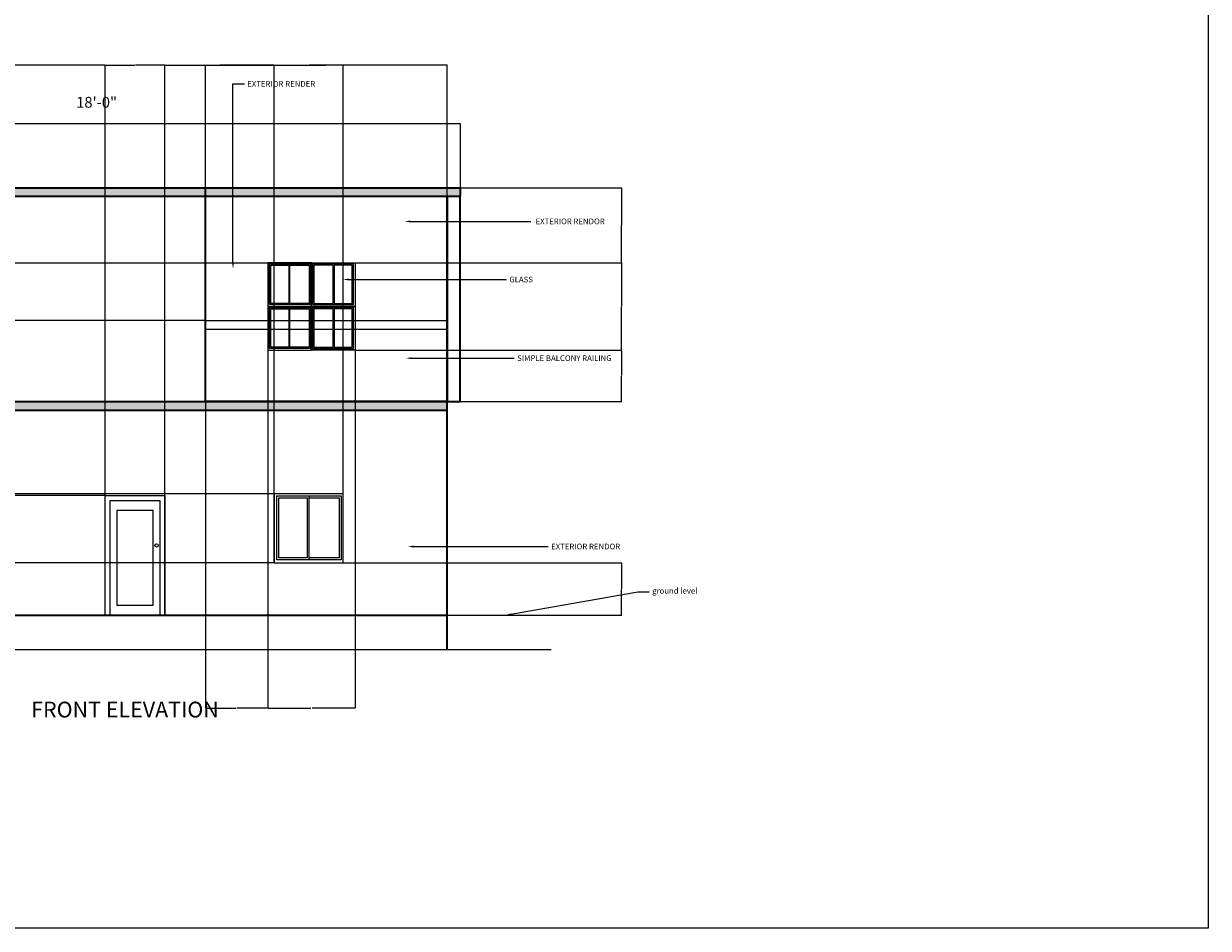
# Model space of a CAD drawing. Units: feet. Extents: x 2813 to 4435, y 1041 to 2557.
# Tile 4 of 6: x 3605 to 4435, y 1041 to 1676. Entities that reach past the tile are written whole.
import ezdxf
from ezdxf import colors
from ezdxf.entities.mleader import LeaderData, LeaderLine
from ezdxf.math import Vec2, Vec3

# ---------------------------------------------------------------- set-up
doc = ezdxf.new("R2010")
doc.units = ezdxf.units.FT
for name, color, linetype, lineweight in [('A-ANNO-DIMS', 2, 'Continuous', 18), ('A-ANNO-SYMB', 7, 'Continuous', 18), ('A-ANNO-TEXT', 7, 'Continuous', 18), ('A-ANNO-TTLB', 7, 'Continuous', 25), ('A-DOOR', 3, 'Continuous', 25), ('A-ELEV', 7, 'Continuous', 35), ('A-ELEV-GRND', 7, 'Continuous', 25), ('A-ELEV-PATT', 252, 'Continuous', 13), ('A-FLOR-HRAL', 4, 'Continuous', 18), ('A-GLAZ', 4, 'Continuous', 18)]:
    doc.layers.add(name, color=color, linetype=linetype, lineweight=lineweight)
doc.styles.get("Standard").update_dxf_attribs({"font": 'arial.ttf'})
doc.dimstyles.get("Standard").update_dxf_attribs({"dimtxt": 0.18, "dimasz": 0.18, "dimexe": 0.18, "dimexo": 0.0625, "dimgap": 0.09, "dimtad": 0, "dimtih": 1, "dimtoh": 1, "dimdec": 4, "dimzin": 0, "dimdsep": 46, "dimtxsty": 'Standard', "dimcen": 0.09, "dimadec": 0, "dimazin": 0, "dimtfac": 1, "dimtdec": 4, "dimtofl": 0, "dimtmove": 0, "dimatfit": 3, "dimfxl": 1, "dimtolj": 1, "dimtzin": 0, "dimarcsym": 0})

# ---------------------------------------------------------------- blocks, each defined once
blk = doc.blocks.new('*U12')
blk.add_lwpolyline([(3.12, 0.01), (0.12, 0.01), (0.12, 72.01), (36.12, 72.01), (36.12, 0.01), (33.12, 0.01)])
for points in [[(33.12, 68.99), (33.12, 0.01), (3.12, 0.01), (3.12, 68.99)], [(29.12, 6.01), (29.12, 62.99), (7.12, 62.99), (7.12, 6.01)]]:
    blk.add_lwpolyline(points, close=True)
blk.add_circle((31.12, 42.01), 1)
blk = doc.blocks.new('*U14')
for p, q in [((38.1, 38.1), (38.1, 876.3)), ((38.1, 876.3), (457.2, 876.3)), ((457.2, 38.1), (457.2, 876.3)), ((457.2, 876.3), (876.3, 876.3)), ((876.3, 876.3), (876.3, 38.1)), ((457.2, 38.1), (38.1, 38.1)), ((876.3, 38.1), (457.2, 38.1))]:
    blk.add_line(p, q)
blk.add_lwpolyline([(0, 0), (900, 0), (900, 900), (0, 900)], close=True)
for points in [[(431.8, 850.9), (431.8, 63.5), (63.5, 63.5), (63.5, 850.9), (431.8, 850.9)], [(457.2, 850.9), (850.9, 850.9), (850.9, 63.5), (457.2, 63.5)]]:
    blk.add_lwpolyline(points)
blk = doc.blocks.new('*D35')
at = {"layer": 'A-ANNO-DIMS', "color": 0, "lineweight": -2, "transparency": 16777216}
for p, q in [((3421.71, 1261.18), (3421.71, 1647.39)), ((3421.89, 1647.21), (3541.42, 1647.21)), ((3661.53, 1647.21), (3542, 1647.21)), ((3661.71, 1261.18), (3661.71, 1647.39))]:
    blk.add_line(p, q, dxfattribs=at)
at = {"layer": 'A-ANNO-DIMS', "color": 0, "transparency": 16777216}
for points in [[(3421.89, 1647.24), (3421.89, 1647.18), (3421.71, 1647.21)], [(3661.53, 1647.24), (3661.53, 1647.18), (3661.71, 1647.21)]]:
    blk.add_solid(points, dxfattribs=at)
at = {"layer": 'DEFPOINTS', "color": 0, "transparency": 16777216}
for p in [(3661.71, 1647.21), (3421.71, 1261.11), (3661.71, 1261.11)]:
    blk.add_point(p, dxfattribs=at)
at = {"layer": 'A-ANNO-DIMS', "color": 0, "transparency": 16777216, "insert": (3541.71, 1647.21), "char_height": 0.18, "attachment_point": 5}
blk.add_mtext('\\A1;240', dxfattribs=at)
blk = doc.blocks.new('*D36')
at = {"layer": 'A-ANNO-DIMS', "color": 0, "lineweight": -2, "transparency": 16777216}
for p, q in [((3661.71, 1345.18), (3661.71, 1647.39)), ((3661.89, 1647.21), (3682.48, 1647.21)), ((3703.53, 1647.21), (3682.93, 1647.21)), ((3703.71, 1345.18), (3703.71, 1647.39))]:
    blk.add_line(p, q, dxfattribs=at)
at = {"layer": 'A-ANNO-DIMS', "color": 0, "transparency": 16777216}
for points in [[(3661.89, 1647.24), (3661.89, 1647.18), (3661.71, 1647.21)], [(3703.53, 1647.24), (3703.53, 1647.18), (3703.71, 1647.21)]]:
    blk.add_solid(points, dxfattribs=at)
at = {"layer": 'DEFPOINTS', "color": 0, "transparency": 16777216}
for p in [(3703.71, 1647.21), (3661.71, 1345.11), (3703.71, 1345.11)]:
    blk.add_point(p, dxfattribs=at)
at = {"layer": 'A-ANNO-DIMS', "color": 0, "transparency": 16777216, "insert": (3682.71, 1647.21), "char_height": 0.18, "attachment_point": 5}
blk.add_mtext('\\A1;42', dxfattribs=at)
blk = doc.blocks.new('*D37')
at = {"layer": 'A-ANNO-DIMS', "color": 0, "lineweight": -2, "transparency": 16777216}
for p, q in [((3703.71, 1261.18), (3703.71, 1647.39)), ((3703.89, 1647.21), (3741.63, 1647.21)), ((3780.03, 1647.21), (3742.28, 1647.21)), ((3780.21, 1297.98), (3780.21, 1647.39))]:
    blk.add_line(p, q, dxfattribs=at)
at = {"layer": 'A-ANNO-DIMS', "color": 0, "transparency": 16777216}
for points in [[(3703.89, 1647.24), (3703.89, 1647.18), (3703.71, 1647.21)], [(3780.03, 1647.24), (3780.03, 1647.18), (3780.21, 1647.21)]]:
    blk.add_solid(points, dxfattribs=at)
at = {"layer": 'DEFPOINTS', "color": 0, "transparency": 16777216}
for p in [(3780.21, 1647.21), (3780.21, 1297.91), (3703.71, 1261.11)]:
    blk.add_point(p, dxfattribs=at)
at = {"layer": 'A-ANNO-DIMS', "color": 0, "transparency": 16777216, "insert": (3741.96, 1647.21), "char_height": 0.18, "attachment_point": 5}
blk.add_mtext('\\A1;76.5', dxfattribs=at)
blk = doc.blocks.new('*D38')
at = {"layer": 'A-ANNO-DIMS', "color": 0, "lineweight": -2, "transparency": 16777216}
for p, q in [((3780.21, 1346.36), (3780.21, 1647.39)), ((3780.39, 1647.21), (3804, 1647.21)), ((3828.4, 1647.21), (3804.79, 1647.21)), ((3828.58, 1346.36), (3828.58, 1647.39))]:
    blk.add_line(p, q, dxfattribs=at)
at = {"layer": 'A-ANNO-DIMS', "color": 0, "transparency": 16777216}
for points in [[(3780.39, 1647.24), (3780.39, 1647.18), (3780.21, 1647.21)], [(3828.4, 1647.24), (3828.4, 1647.18), (3828.58, 1647.21)]]:
    blk.add_solid(points, dxfattribs=at)
at = {"layer": 'DEFPOINTS', "color": 0, "transparency": 16777216}
for p in [(3828.58, 1647.21), (3780.21, 1346.29), (3828.58, 1346.29)]:
    blk.add_point(p, dxfattribs=at)
at = {"layer": 'A-ANNO-DIMS', "color": 0, "transparency": 16777216, "insert": (3804.39, 1647.21), "char_height": 0.18, "attachment_point": 5}
blk.add_mtext('\\A1;48.38', dxfattribs=at)
blk = doc.blocks.new('*D41')
at = {"layer": 'A-ANNO-DIMS', "color": 0, "lineweight": -2, "transparency": 16777216}
for p, q in [((3775.79, 1447.05), (3775.79, 1195.88)), ((3732.18, 1411.05), (3732.18, 1195.88)), ((3732.36, 1196.06), (3753.61, 1196.06)), ((3775.61, 1196.06), (3754.37, 1196.06))]:
    blk.add_line(p, q, dxfattribs=at)
at = {"layer": 'A-ANNO-DIMS', "color": 0, "transparency": 16777216}
for points in [[(3732.36, 1196.09), (3732.36, 1196.03), (3732.18, 1196.06)], [(3775.61, 1196.09), (3775.61, 1196.03), (3775.79, 1196.06)]]:
    blk.add_solid(points, dxfattribs=at)
at = {"layer": 'DEFPOINTS', "color": 0, "transparency": 16777216}
for p in [(3775.79, 1447.11), (3732.18, 1411.11), (3775.79, 1196.06)]:
    blk.add_point(p, dxfattribs=at)
at = {"layer": 'A-ANNO-DIMS', "color": 0, "transparency": 16777216, "insert": (3753.99, 1196.06), "char_height": 0.18, "attachment_point": 5}
blk.add_mtext('\\A1;43.61', dxfattribs=at)
blk = doc.blocks.new('*D42')
at = {"layer": 'A-ANNO-DIMS', "color": 0, "lineweight": -2, "transparency": 16777216}
for p, q in [((3775.79, 1447.05), (3775.79, 1195.88)), ((3837.14, 1447.05), (3837.14, 1195.88)), ((3775.97, 1196.06), (3806.07, 1196.06)), ((3836.96, 1196.06), (3806.86, 1196.06))]:
    blk.add_line(p, q, dxfattribs=at)
at = {"layer": 'A-ANNO-DIMS', "color": 0, "transparency": 16777216}
for points in [[(3775.97, 1196.09), (3775.97, 1196.03), (3775.79, 1196.06)], [(3836.96, 1196.09), (3836.96, 1196.03), (3837.14, 1196.06)]]:
    blk.add_solid(points, dxfattribs=at)
at = {"layer": 'DEFPOINTS', "color": 0, "transparency": 16777216}
for p in [(3775.79, 1447.11), (3837.14, 1447.11), (3837.14, 1196.06)]:
    blk.add_point(p, dxfattribs=at)
at = {"layer": 'A-ANNO-DIMS', "color": 0, "transparency": 16777216, "insert": (3806.46, 1196.06), "char_height": 0.18, "attachment_point": 5}
blk.add_mtext('\\A1;61.35', dxfattribs=at)
blk = doc.blocks.new('*D43')
at = {"layer": 'A-ANNO-DIMS', "color": 0, "lineweight": -2, "transparency": 16777216}
for p, q in [((3661.64, 1345.11), (3260.3, 1345.11)), ((3260.48, 1344.93), (3260.48, 1303.3)), ((3260.48, 1261.29), (3260.48, 1302.93)), ((3661.64, 1261.11), (3260.3, 1261.11))]:
    blk.add_line(p, q, dxfattribs=at)
at = {"layer": 'A-ANNO-DIMS', "color": 0, "transparency": 16777216}
for points in [[(3260.45, 1344.93), (3260.51, 1344.93), (3260.48, 1345.11)], [(3260.45, 1261.29), (3260.51, 1261.29), (3260.48, 1261.11)]]:
    blk.add_solid(points, dxfattribs=at)
at = {"layer": 'DEFPOINTS', "color": 0, "transparency": 16777216}
for p in [(3260.48, 1345.11), (3661.71, 1345.11), (3661.71, 1261.11)]:
    blk.add_point(p, dxfattribs=at)
at = {"layer": 'A-ANNO-DIMS', "color": 0, "transparency": 16777216, "insert": (3260.48, 1303.11), "char_height": 0.18, "attachment_point": 5}
blk.add_mtext('\\A1;84', dxfattribs=at)
blk = doc.blocks.new('*D44')
at = {"layer": 'A-ANNO-DIMS', "color": 0, "lineweight": -2, "transparency": 16777216}
for p, q in [((3780.27, 1297.91), (4024.11, 1297.91)), ((4023.93, 1297.73), (4023.93, 1279.7)), ((4023.93, 1261.29), (4023.93, 1279.33)), ((3703.77, 1261.11), (4024.11, 1261.11))]:
    blk.add_line(p, q, dxfattribs=at)
at = {"layer": 'A-ANNO-DIMS', "color": 0, "transparency": 16777216}
for points in [[(4023.9, 1297.73), (4023.96, 1297.73), (4023.93, 1297.91)], [(4023.9, 1261.29), (4023.96, 1261.29), (4023.93, 1261.11)]]:
    blk.add_solid(points, dxfattribs=at)
at = {"layer": 'DEFPOINTS', "color": 0, "transparency": 16777216}
for p in [(3780.21, 1297.91), (4023.93, 1297.91), (3703.71, 1261.11)]:
    blk.add_point(p, dxfattribs=at)
at = {"layer": 'A-ANNO-DIMS', "color": 0, "transparency": 16777216, "insert": (4023.93, 1279.51), "char_height": 0.18, "attachment_point": 5}
blk.add_mtext('\\A1;36.8', dxfattribs=at)
blk = doc.blocks.new('*D45')
at = {"layer": 'A-ANNO-DIMS', "color": 0, "lineweight": -2, "transparency": 16777216}
for p, q in [((3780.14, 1346.29), (3260.3, 1346.29)), ((3260.48, 1346.11), (3260.48, 1322.29)), ((3260.48, 1298.09), (3260.48, 1321.92)), ((3780.14, 1297.91), (3260.3, 1297.91))]:
    blk.add_line(p, q, dxfattribs=at)
at = {"layer": 'A-ANNO-DIMS', "color": 0, "transparency": 16777216}
for points in [[(3260.45, 1346.11), (3260.51, 1346.11), (3260.48, 1346.29)], [(3260.45, 1298.09), (3260.51, 1298.09), (3260.48, 1297.91)]]:
    blk.add_solid(points, dxfattribs=at)
at = {"layer": 'DEFPOINTS', "color": 0, "transparency": 16777216}
for p in [(3260.48, 1346.29), (3780.21, 1346.29), (3780.21, 1297.91)]:
    blk.add_point(p, dxfattribs=at)
at = {"layer": 'A-ANNO-DIMS', "color": 0, "transparency": 16777216, "insert": (3260.48, 1322.1), "char_height": 0.18, "attachment_point": 5}
blk.add_mtext('\\A1;48.38', dxfattribs=at)
blk = doc.blocks.new('*D47')
at = {"layer": 'A-ANNO-DIMS', "color": 0, "lineweight": -2, "transparency": 16777216}
for p, q in [((3421.77, 1561.11), (4024.11, 1561.11)), ((4023.93, 1560.93), (4023.93, 1534.97)), ((4023.93, 1508.64), (4023.93, 1534.61)), ((3480.84, 1508.46), (4024.11, 1508.46))]:
    blk.add_line(p, q, dxfattribs=at)
at = {"layer": 'A-ANNO-DIMS', "color": 0, "transparency": 16777216}
for points in [[(4023.9, 1560.93), (4023.96, 1560.93), (4023.93, 1561.11)], [(4023.9, 1508.64), (4023.96, 1508.64), (4023.93, 1508.46)]]:
    blk.add_solid(points, dxfattribs=at)
at = {"layer": 'DEFPOINTS', "color": 0, "transparency": 16777216}
for p in [(3421.71, 1561.11), (3480.78, 1508.46), (4023.93, 1508.46)]:
    blk.add_point(p, dxfattribs=at)
at = {"layer": 'A-ANNO-DIMS', "color": 0, "transparency": 16777216, "insert": (4023.93, 1534.79), "char_height": 0.18, "attachment_point": 5}
blk.add_mtext('\\A1;52.65', dxfattribs=at)
blk = doc.blocks.new('*D48')
at = {"layer": 'A-ANNO-DIMS', "color": 0, "lineweight": -2, "transparency": 16777216}
for p, q in [((3837.2, 1508.46), (4024.11, 1508.46)), ((4023.93, 1508.28), (4023.93, 1477.97)), ((4023.93, 1447.29), (4023.93, 1477.61)), ((3837.2, 1447.11), (4024.11, 1447.11))]:
    blk.add_line(p, q, dxfattribs=at)
at = {"layer": 'A-ANNO-DIMS', "color": 0, "transparency": 16777216}
for points in [[(4023.9, 1508.28), (4023.96, 1508.28), (4023.93, 1508.46)], [(4023.9, 1447.29), (4023.96, 1447.29), (4023.93, 1447.11)]]:
    blk.add_solid(points, dxfattribs=at)
at = {"layer": 'DEFPOINTS', "color": 0, "transparency": 16777216}
for p in [(3837.14, 1508.46), (4023.93, 1508.46), (3837.14, 1447.11)]:
    blk.add_point(p, dxfattribs=at)
at = {"layer": 'A-ANNO-DIMS', "color": 0, "transparency": 16777216, "insert": (4023.93, 1477.79), "char_height": 0.18, "attachment_point": 5}
blk.add_mtext('\\A1;61.35', dxfattribs=at)
blk = doc.blocks.new('*D49')
at = {"layer": 'A-ANNO-DIMS', "color": 0, "lineweight": -2, "transparency": 16777216}
for p, q in [((3732.12, 1467.89), (3260.3, 1467.89)), ((3260.48, 1467.71), (3260.48, 1439.68)), ((3260.48, 1411.29), (3260.48, 1439.32)), ((3732.12, 1411.11), (3260.3, 1411.11))]:
    blk.add_line(p, q, dxfattribs=at)
at = {"layer": 'A-ANNO-DIMS', "color": 0, "transparency": 16777216}
for points in [[(3260.45, 1467.71), (3260.51, 1467.71), (3260.48, 1467.89)], [(3260.45, 1411.29), (3260.51, 1411.29), (3260.48, 1411.11)]]:
    blk.add_solid(points, dxfattribs=at)
at = {"layer": 'DEFPOINTS', "color": 0, "transparency": 16777216}
for p in [(3260.48, 1467.89), (3732.18, 1467.89), (3732.18, 1411.11)]:
    blk.add_point(p, dxfattribs=at)
at = {"layer": 'A-ANNO-DIMS', "color": 0, "transparency": 16777216, "insert": (3260.48, 1439.5), "char_height": 0.18, "attachment_point": 5}
blk.add_mtext('\\A1;56.77', dxfattribs=at)
blk = doc.blocks.new('*D50')
at = {"layer": 'A-ANNO-DIMS', "color": 0, "lineweight": -2, "transparency": 16777216}
for p, q in [((3837.2, 1447.11), (4024.11, 1447.11)), ((4023.93, 1446.93), (4023.93, 1429.3)), ((4023.93, 1411.29), (4023.93, 1428.93)), ((3901.77, 1411.11), (4024.11, 1411.11))]:
    blk.add_line(p, q, dxfattribs=at)
at = {"layer": 'A-ANNO-DIMS', "color": 0, "transparency": 16777216}
for points in [[(4023.9, 1446.93), (4023.96, 1446.93), (4023.93, 1447.11)], [(4023.9, 1411.29), (4023.96, 1411.29), (4023.93, 1411.11)]]:
    blk.add_solid(points, dxfattribs=at)
at = {"layer": 'DEFPOINTS', "color": 0, "transparency": 16777216}
for p in [(3837.14, 1447.11), (4023.93, 1447.11), (3901.71, 1411.11)]:
    blk.add_point(p, dxfattribs=at)
at = {"layer": 'A-ANNO-DIMS', "color": 0, "transparency": 16777216, "insert": (4023.93, 1429.11), "char_height": 0.18, "attachment_point": 5}
blk.add_mtext('\\A1;36', dxfattribs=at)
blk = doc.blocks.new('*D51')
at = {"layer": 'A-ANNO-DIMS', "color": 0, "lineweight": -2, "transparency": 16777216}
for p, q in [((3732.18, 1411.18), (3732.18, 1647.39)), ((3732.36, 1647.21), (3816.49, 1647.21)), ((3901.53, 1647.21), (3817.4, 1647.21)), ((3901.71, 1411.18), (3901.71, 1647.39))]:
    blk.add_line(p, q, dxfattribs=at)
at = {"layer": 'A-ANNO-DIMS', "color": 0, "transparency": 16777216}
for points in [[(3732.36, 1647.24), (3732.36, 1647.18), (3732.18, 1647.21)], [(3901.53, 1647.24), (3901.53, 1647.18), (3901.71, 1647.21)]]:
    blk.add_solid(points, dxfattribs=at)
at = {"layer": 'DEFPOINTS', "color": 0, "transparency": 16777216}
for p in [(3901.71, 1647.21), (3732.18, 1411.11), (3901.71, 1411.11)]:
    blk.add_point(p, dxfattribs=at)
at = {"layer": 'A-ANNO-DIMS', "color": 0, "transparency": 16777216, "insert": (3816.94, 1647.21), "char_height": 0.18, "attachment_point": 5}
blk.add_mtext('\\A1;169.52', dxfattribs=at)

msp = doc.modelspace()

# ---------------------------------------------------------------- hatches: boundary and pattern name
at = {"layer": 'A-ELEV-PATT'}
h = msp.add_hatch(color=256, dxfattribs=at)
h.dxf.hatch_style = 1
h.paths.add_polyline_path([(3732.181, 1561.114), (3421.706, 1561.114), (3421.706, 1555.114), (3732.181, 1555.114)])
h.paths.add_polyline_path([(3910.706, 1561.114), (3901.706, 1561.114), (3751.395, 1561.114), (3751.395, 1555.114), (3901.706, 1555.114), (3910.706, 1555.114)])
h.paths.add_polyline_path([(3751.395, 1561.114), (3732.181, 1561.114), (3732.181, 1555.114), (3751.395, 1555.114)])
h.paths.add_polyline_path([(3421.706, 1561.114), (3374.104, 1561.114), (3374.104, 1555.114), (3421.706, 1555.114)])
h.paths.add_polyline_path([(3901.706, 1411.114), (3732.181, 1411.114), (3421.706, 1411.114), (3421.706, 1405.114), (3901.706, 1405.114)])
h.paths.add_polyline_path([(3421.706, 1411.114), (3374.104, 1411.114), (3374.104, 1405.114), (3421.706, 1405.114)])

# ---------------------------------------------------------------- linework, layer by layer
at = {"layer": 'A-ANNO-DIMS'}
for p, q in [((3374.104, 1606.165), (3910.706, 1606.165)), ((3910.706, 1606.165), (3910.706, 1561.114))]:
    msp.add_line(p, q, dxfattribs=at)
at = {"layer": 'A-ANNO-TTLB'}
for p, q in [((4435.474, 2556.562), (4435.474, 1041.465)), ((4435.474, 1041.465), (2933.466, 1041.465))]:
    msp.add_line(p, q, dxfattribs=at)
at = {"layer": 'A-ELEV'}
for p, q in [((3350.104, 1561.114), (3901.706, 1561.114)), ((3374.104, 1555.114), (3901.706, 1555.114)), ((3732.181, 1555.114), (3732.181, 1561.114)), ((3901.706, 1561.114), (3910.706, 1561.114)), ((3901.706, 1237.114), (3901.706, 1555.114)), ((3901.706, 1411.114), (3901.706, 1555.114)), ((3901.706, 1555.114), (3910.706, 1555.114)), ((3910.706, 1561.114), (3910.706, 1555.114)), ((3910.706, 1411.114), (3910.706, 1555.114)), ((3374.104, 1411.114), (3910.706, 1411.114)), ((3374.104, 1405.114), (3901.706, 1405.114)), ((3421.706, 1261.114), (3901.706, 1261.114))]:
    msp.add_line(p, q, dxfattribs=at)
msp.add_lwpolyline([(3732.181, 1555.114), (3901.706, 1555.114), (3901.706, 1411.114), (3732.181, 1411.114)], close=True, dxfattribs=at)
at = {"layer": 'A-ELEV-GRND'}
for p, q in [((3901.706, 1261.114), (3982.882, 1261.114)), ((3421.706, 1237.114), (3901.706, 1237.114)), ((3901.706, 1237.114), (3974.556, 1237.114))]:
    msp.add_line(p, q, dxfattribs=at)
at = {"layer": 'A-FLOR-HRAL'}
for p, q in [((3732.181, 1467.886), (3901.706, 1467.886)), ((3732.181, 1461.886), (3901.706, 1461.886))]:
    msp.add_line(p, q, dxfattribs=at)

# ---------------------------------------------------------------- block references
at = {"layer": 'A-DOOR', "xscale": 1.166666666666666, "yscale": 1.166666666666666, "zscale": 1.166666666666666}
msp.add_blockref('*U12', (3661.562, 1261.099), dxfattribs=at)
at = {"layer": 'A-GLAZ'}
for p, xscale, yscale, zscale in [((3775.791, 1477.788), 0.0340819276308726, 0.0340819276308726, 0.0340819276308726), ((3837.138, 1477.788), -0.0340819276308726, 0.0340819276308726, 0.0340819276308726), ((3775.791, 1447.114), 0.0340819276308726, 0.0340819276308726, 0.0340819276308726), ((3837.138, 1447.114), -0.0340819276308726, 0.0340819276308726, 0.0340819276308726), ((3780.205, 1297.915), 0.0537544395331253, 0.0537544395331253, 0.0537544395331253)]:
    msp.add_blockref('*U14', p, dxfattribs=dict(at, xscale=xscale, yscale=yscale, zscale=zscale))

# ---------------------------------------------------------------- texts
at = {"layer": 'A-ANNO-DIMS', "insert": (3641.405, 1624.886), "char_height": 7.6018, "attachment_point": 1}
msp.add_mtext_dynamic_manual_height_columns('18\'-0"', width=61.91074, gutter_width=38.009, heights=[0], dxfattribs=at)
at = {"layer": 'A-ANNO-TEXT', "insert": (3609.833, 1200.48), "char_height": 11.04352, "attachment_point": 1}
msp.add_mtext_dynamic_manual_height_columns('FRONT ELEVATION', width=1286.33739, gutter_width=55.218, heights=[0], dxfattribs=at)

# ---------------------------------------------------------------- dimensions: what is measured, and where the dimension line sits
at = {"layer": 'A-ANNO-DIMS'}
for base, p1, p2, override, picture, middle in [((3661.706, 1647.215), (3421.706, 1261.114), (3661.706, 1261.114), {"dimdec": 0, "dimlfac": 1, "dimrnd": 0, "dimzin": 0, "dimdsep": 46, "dimlunit": 2}, '*D35', (3541.706, 1647.215)), ((3703.706, 1647.215), (3661.706, 1345.114), (3703.706, 1345.114), {"dimdec": 0, "dimlfac": 1, "dimrnd": 0, "dimzin": 0, "dimdsep": 46, "dimlunit": 2}, '*D36', (3682.706, 1647.215)), ((3780.205, 1647.215), (3703.706, 1261.114), (3780.205, 1297.915), {"dimdec": 1, "dimlfac": 1, "dimrnd": 0, "dimzin": 0, "dimdsep": 46, "dimlunit": 2}, '*D37', (3741.956, 1647.215)), ((3901.70615, 1647.21469), (3732.18117, 1411.1143), (3901.70615, 1411.1143), {"dimdec": 2, "dimlfac": 1, "dimrnd": 0, "dimzin": 0, "dimdsep": 46, "dimlunit": 2}, '*D51', (3816.94366, 1647.21469)), ((3828.584, 1647.215), (3780.205, 1346.294), (3828.584, 1346.294), {"dimdec": 2, "dimlfac": 1, "dimrnd": 0, "dimzin": 0, "dimdsep": 46, "dimlunit": 2}, '*D38', (3804.395, 1647.215)), ((3775.791, 1196.064), (3732.181, 1411.114), (3775.791, 1447.114), {"dimdec": 2, "dimlfac": 1, "dimrnd": 0, "dimzin": 0, "dimdsep": 46, "dimlunit": 2}, '*D41', (3753.986, 1196.064)), ((3837.138, 1196.064), (3775.791, 1447.114), (3837.138, 1447.114), {"dimdec": 2, "dimlfac": 1, "dimrnd": 0, "dimzin": 0, "dimdsep": 46, "dimlunit": 2}, '*D42', (3806.464, 1196.064))]:
    dim = msp.add_linear_dim(base=base, p1=p1, p2=p2, dimstyle='Standard', override=override, dxfattribs=at)
    dim.commit()
    dim.dimension.update_dxf_attribs({"geometry": picture, "text_midpoint": middle})
for base, p1, p2, override, picture, middle in [((4023.932, 1508.462), (3421.706, 1561.114), (3480.779, 1508.462), {"dimdec": 2, "dimlfac": 1, "dimrnd": 0, "dimzin": 0, "dimdsep": 46, "dimlunit": 2}, '*D47', (4023.932, 1534.788)), ((4023.932, 1508.462), (3837.138, 1447.114), (3837.138, 1508.462), {"dimdec": 2, "dimlfac": 1, "dimrnd": 0, "dimzin": 0, "dimdsep": 46, "dimlunit": 2}, '*D48', (4023.932, 1477.788)), ((3260.476, 1467.886), (3732.181, 1411.114), (3732.181, 1467.886), {"dimdec": 2, "dimlfac": 1, "dimrnd": 0, "dimzin": 0, "dimdsep": 46, "dimlunit": 2}, '*D49', (3260.476, 1439.5)), ((4023.932, 1447.114), (3901.706, 1411.114), (3837.138, 1447.114), {"dimdec": 0, "dimlfac": 1, "dimrnd": 0, "dimzin": 0, "dimdsep": 46, "dimlunit": 2}, '*D50', (4023.932, 1429.114)), ((3260.476, 1346.294), (3780.205, 1297.915), (3780.205, 1346.294), {"dimdec": 2, "dimlfac": 1, "dimrnd": 0, "dimzin": 0, "dimdsep": 46, "dimlunit": 2}, '*D45', (3260.476, 1322.104)), ((3260.476, 1345.114), (3661.706, 1261.114), (3661.706, 1345.114), {"dimdec": 0, "dimlfac": 1, "dimrnd": 0, "dimzin": 0, "dimdsep": 46, "dimlunit": 2}, '*D43', (3260.476, 1303.114)), ((4023.932, 1297.915), (3703.706, 1261.114), (3780.205, 1297.915), {"dimdec": 1, "dimlfac": 1, "dimrnd": 0, "dimzin": 0, "dimdsep": 46, "dimlunit": 2}, '*D44', (4023.932, 1279.514))]:
    dim = msp.add_linear_dim(base=base, p1=p1, p2=p2, angle=90, dimstyle='Standard', override=override, dxfattribs=at)
    dim.commit()
    dim.dimension.update_dxf_attribs({"geometry": picture, "text_midpoint": middle})

# ---------------------------------------------------------------- leaders
at = {"layer": 'A-ANNO-SYMB'}
ml = msp.add_multileader_mtext('Standard', dxfattribs=at)
ml.set_content('ground level', color=256)
ml.set_leader_properties()
ml.build(insert=Vec2(0, 0))
ctx = ml.context
ctx.base_point, ctx.plane_origin = Vec3(4043.415, 1277.694), Vec3(3942.294, 1261.114)
notes = []
notes.append((ctx, [(0, (1, 1, 0), (4035.415, 1277.694), (1, 0), 8, [(0, [(3942.294, 1261.114)], 0, [])])]))
ctx.mtext.insert, ctx.mtext.flow_direction = Vec3(4045.415, 1280.282), 5
at = {"layer": 'A-ANNO-TEXT'}
ml = msp.add_multileader_mtext('Standard', dxfattribs=at)
ml.set_content('EXTERIOR RENDER', color=256)
ml.set_leader_properties()
ml.build(insert=Vec2(0, 0))
ctx = ml.context
ctx.base_point, ctx.plane_origin = Vec3(3759.395, 1633.985), Vec3(3751.395, 1504.33)
notes.append((ctx, [(0, (1, 1, 0), (3751.395, 1633.985), (1, 0), 8, [(0, [(3751.395, 1504.33)], 0, [])])]))
ctx.mtext.insert, ctx.mtext.flow_direction = Vec3(3761.395, 1636.019), 5
ml = msp.add_multileader_mtext('Standard', dxfattribs=at)
ml.set_content(' EXTERIOR RENDOR', color=256)
ml.set_leader_properties()
ml.build(insert=Vec2(0, 0))
ctx = ml.context
ctx.base_point, ctx.plane_origin = Vec3(3960.376, 1537.496), Vec3(3871.791, 1537.496)
notes.append((ctx, [(0, (1, 1, 0), (3952.376, 1537.496), (1, 0), 8, [(0, [(3871.791, 1537.496)], 0, [])])]))
ctx.mtext.insert, ctx.mtext.flow_direction = Vec3(3962.376, 1539.53), 5
ml = msp.add_multileader_mtext('Standard', dxfattribs=at)
ml.set_content('GLASS', color=256)
ml.set_leader_properties()
ml.build(insert=Vec2(0, 0))
ctx = ml.context
ctx.base_point, ctx.plane_origin = Vec3(3943.23, 1496.715), Vec3(3828.584, 1496.715)
notes.append((ctx, [(0, (1, 1, 0), (3935.23, 1496.715), (1, 0), 8, [(0, [(3828.584, 1496.715)], 0, [])])]))
ctx.mtext.insert, ctx.mtext.flow_direction = Vec3(3945.23, 1498.749), 5
ml = msp.add_multileader_mtext('Standard', dxfattribs=at)
ml.set_content('SIMPLE BALCONY RAILING', color=256)
ml.set_leader_properties()
ml.build(insert=Vec2(0, 0))
ctx = ml.context
ctx.base_point, ctx.plane_origin = Vec3(3948.717, 1441.54), Vec3(3872.82, 1441.54)
notes.append((ctx, [(0, (1, 1, 0), (3940.717, 1441.54), (1, 0), 8, [(0, [(3872.82, 1441.54)], 0, [])])]))
ctx.mtext.insert, ctx.mtext.flow_direction = Vec3(3950.717, 1443.574), 5
ml = msp.add_multileader_mtext('Standard', dxfattribs=at)
ml.set_content('EXTERIOR RENDOR', color=256)
ml.set_leader_properties()
ml.build(insert=Vec2(0, 0))
ctx = ml.context
ctx.base_point, ctx.plane_origin = Vec3(3972.504, 1309.339), Vec3(3874.014, 1309.339)
notes.append((ctx, [(0, (1, 1, 0), (3964.504, 1309.339), (1, 0), 8, [(0, [(3874.014, 1309.339)], 0, [])])]))
ctx.mtext.insert, ctx.mtext.flow_direction = Vec3(3974.504, 1311.373), 5
for ctx, leaders in notes:
    for number, flags, end, landing, length, lines in leaders:
        leader = LeaderData()
        leader.index, (leader.has_last_leader_line, leader.has_dogleg_vector, leader.attachment_direction) = number, flags
        leader.last_leader_point, leader.dogleg_vector, leader.dogleg_length = Vec3(end), Vec3(landing), length
        for number, points, colour, breaks in lines:
            line = LeaderLine()
            line.index, line.vertices, line.color, line.breaks = number, Vec3.list(points), colors.encode_raw_color(colour), breaks
            leader.lines.append(line)
        ctx.leaders.append(leader)

doc.saveas('drawing.dxf')
